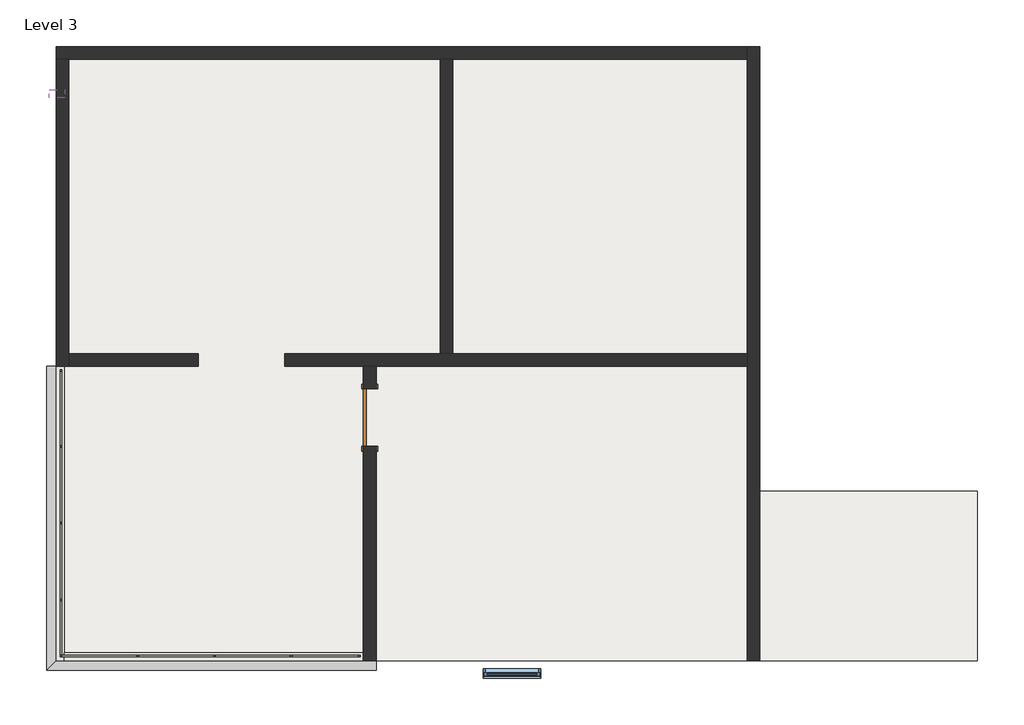
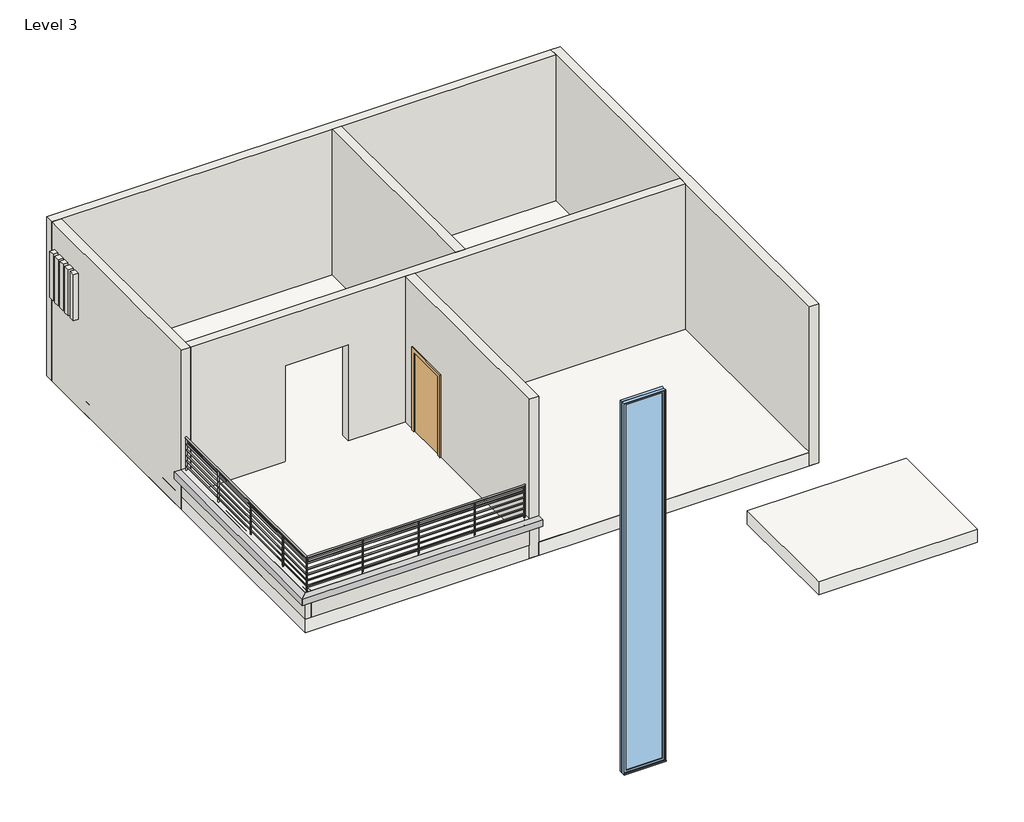
# One storey: 9 walls, 4 roofs, 2 proxies, 1 door, 1 railing, 1 window.
"""IFC4 building model written with IfcOpenShell, lengths in millimetres."""

from ifc_helpers import new_model, si_unit, point, frame, frame_2d, origin, place, context, project, spatial, polyline, circle_curve, ellipse_curve, trimmed, segment, composite_curve, outline, extrude, faceted_brep, transform, mapped, element, save
from ifc_brep_helpers import plane_surface, cylinder_surface, advanced_brep
from components import door_54dd4da4, walls_4_walls_4_d362682a, window_9b859ad1

model = new_model("IFC4")

# Units and contexts
model_context = context("Model", 3, world=origin())
ifc_project = project(units=[si_unit("LENGTHUNIT", "METRE", prefix="MILLI")], contexts=[model_context])

# Site, building, storey
site = spatial("IfcSite", under=ifc_project)
building = spatial("IfcBuilding", under=site)
storey = spatial("IfcBuildingStorey", under=building, Name="Level 3", Elevation=7315.2)

# Proxies
placement = place(None, origin())
element("IfcBuildingElementProxy", 1, Name="Cornice", ObjectType="Cornice", at=placement, inside=storey, context=model_context, shape_type="SweptSolid", body=[
    extrude(outline(polyline([(-12708.8681702, 4224.2612165), (-12556.4681702, 4224.2612165), (-12556.4681702, -449.3387835), (-12708.8681702, -601.7387835), (-12708.8681702, 4224.2612165)])), frame((0.0, 0.0, 8077.2), z_axis=(0.0, 0.0, 1.0), x_axis=(1.0, 0.0, 0.0)), (0.0, 0.0, 1.0), 152.4),
])
element("IfcBuildingElementProxy", 2, Name="Cornice", ObjectType="Cornice", at=placement, inside=storey, context=model_context, shape_type="SweptSolid", body=[
    extrude(outline(polyline([(-12708.8681702, -601.7387835), (-12556.4681702, -449.3387835), (-7476.4681702, -449.3387835), (-7476.4681702, -601.7387835), (-12708.8681702, -601.7387835)])), frame((0.0, 0.0, 8077.2), z_axis=(0.0, 0.0, 1.0), x_axis=(1.0, 0.0, 0.0)), (0.0, 0.0, 1.0), 152.4),
])

# Door
door_shape = door_54dd4da4(model_context)
element("IfcDoor", 3, ObjectType="Single-Flush : 36\" x 84\"", at=placement, inside=storey, context=model_context, shape_type="MappedRepresentation", body=[
    mapped(door_shape, transform((-7578.0681702, 3411.4612165, 7315.2), x_axis=(0.0, 1.0, 0.0), y_axis=(-1.0, 0.0, 0.0), z_axis=(0.0, 0.0, 1.0))),
])

# Railing
element("IfcRailing", 4, ObjectType="Guardrail - Pipe", at=placement, inside=storey, context=model_context, shape_type="SolidModel", body=[
    advanced_brep(
    [(-12423.1181702, 4173.4612165, 8820.15), (-12385.0181702, 4173.4612165, 8820.15), (-12423.1181702, -315.9887835, 8820.15), (-12385.0181702, -277.8887835, 8820.15), (-7730.4681702, -315.9887835, 8820.15), (-7730.4681702, -277.8887835, 8820.15)],
    [
        (0, 1, circle_curve(frame((-12404.0681702, 4173.4612165, 8820.15), z_axis=(0.0, 1.0, 0.0), x_axis=(1.0, 0.0, 0.0)), 19.05)),
        (1, 0, circle_curve(frame((-12404.0681702, 4173.4612165, 8820.15), z_axis=(0.0, 1.0, 0.0), x_axis=(1.0, 0.0, 0.0)), 19.05)),
        (0, 2),
        (2, 3, ellipse_curve(frame((-12404.0681702, -296.9387835, 8820.15), z_axis=(-0.7071067811865459, 0.7071067811865492, 0.0), x_axis=(0.7071067811865492, 0.7071067811865458, 0.0)), 26.9407684, 19.05)),
        (3, 1),
        (3, 2, ellipse_curve(frame((-12404.0681702, -296.9387835, 8820.15), z_axis=(-0.7071067811865459, 0.7071067811865492, 0.0), x_axis=(0.7071067811865492, 0.7071067811865458, 0.0)), 26.9407684, 19.05)),
        (4, 5, circle_curve(frame((-7730.4681702, -296.9387835, 8820.15), z_axis=(1.0, 0.0, 0.0), x_axis=(0.0, 1.0, 0.0)), 19.05)),
        (5, 4, circle_curve(frame((-7730.4681702, -296.9387835, 8820.15), z_axis=(1.0, 0.0, 0.0), x_axis=(0.0, 1.0, 0.0)), 19.05)),
        (2, 4),
        (5, 3),
    ],
    [
        plane_surface(frame((-12404.0681702, 4173.4612165, 8839.2), z_axis=(0.0, 1.0, 0.0), x_axis=(0.0, 0.0, -1.0))),
        cylinder_surface(frame((-12404.0681702, 4173.4612165, 8820.15), z_axis=(0.0, 1.0, 0.0), x_axis=(1.0, 0.0, 0.0)), 19.05),
        plane_surface(frame((-7730.4681702, -296.9387835, 8839.2), z_axis=(1.0, 0.0, 0.0), x_axis=(0.0, 1.0, 0.0))),
        cylinder_surface(frame((-12404.0681702, -296.9387835, 8820.15), z_axis=(-1.0, 0.0, 0.0), x_axis=(0.0, 1.0, 0.0)), 19.05),
    ],
    [
        (0, [[1, 2]]),
        (1, [[-1, 3, 4, 5]]),
        (1, [[-2, -5, 6, -3]]),
        (2, [[7, 8]]),
        (3, [[-4, 9, -8, 10]]),
        (3, [[-6, -10, -7, -9]]),
    ],
),
    advanced_brep(
    [(-12499.3181702, 4173.4612165, 8972.55), (-12461.2181702, 4173.4612165, 8972.55), (-7730.4681702, -392.1887835, 8972.55), (-7730.4681702, -354.0887835, 8972.55), (-12499.3181702, -392.1887835, 8972.55), (-12461.2181702, -354.0887835, 8972.55)],
    [
        (0, 1, circle_curve(frame((-12480.2681702, 4173.4612165, 8972.55), z_axis=(0.0, 1.0, 0.0), x_axis=(1.0, 0.0, 0.0)), 19.05)),
        (1, 0, circle_curve(frame((-12480.2681702, 4173.4612165, 8972.55), z_axis=(0.0, 1.0, 0.0), x_axis=(1.0, 0.0, 0.0)), 19.05)),
        (2, 3, circle_curve(frame((-7730.4681702, -373.1387835, 8972.55), z_axis=(1.0, 0.0, 0.0), x_axis=(0.0, 1.0, 0.0)), 19.05)),
        (3, 2, circle_curve(frame((-7730.4681702, -373.1387835, 8972.55), z_axis=(1.0, 0.0, 0.0), x_axis=(0.0, 1.0, 0.0)), 19.05)),
        (0, 4),
        (4, 5, ellipse_curve(frame((-12480.2681702, -373.1387835, 8972.55), z_axis=(-0.7071067811865459, 0.7071067811865492, 0.0), x_axis=(0.7071067811865492, 0.7071067811865458, 0.0)), 26.9407684, 19.05)),
        (5, 1),
        (5, 4, ellipse_curve(frame((-12480.2681702, -373.1387835, 8972.55), z_axis=(-0.7071067811865459, 0.7071067811865492, 0.0), x_axis=(0.7071067811865492, 0.7071067811865458, 0.0)), 26.9407684, 19.05)),
        (4, 2),
        (3, 5),
    ],
    [
        plane_surface(frame((-12480.2681702, 4173.4612165, 8991.6), z_axis=(0.0, 1.0, 0.0), x_axis=(0.0, 0.0, -1.0))),
        plane_surface(frame((-7730.4681702, -373.1387835, 8991.6), z_axis=(1.0, 0.0, 0.0), x_axis=(0.0, 1.0, 0.0))),
        cylinder_surface(frame((-12480.2681702, 4173.4612165, 8972.55), z_axis=(0.0, 1.0, 0.0), x_axis=(1.0, 0.0, 0.0)), 19.05),
        cylinder_surface(frame((-12480.2681702, -373.1387835, 8972.55), z_axis=(-1.0, 0.0, 0.0), x_axis=(0.0, 1.0, 0.0)), 19.05),
    ],
    [
        (0, [[1, 2]]),
        (1, [[3, 4]]),
        (2, [[-1, 5, 6, 7]]),
        (2, [[-2, -7, 8, -5]]),
        (3, [[-6, 9, -4, 10]]),
        (3, [[-8, -10, -3, -9]]),
    ],
),
    advanced_brep(
    [(-12467.5681702, 4173.4612165, 8826.5), (-12492.9681702, 4173.4612165, 8826.5), (-7730.4681702, -360.4387835, 8826.5), (-7730.4681702, -385.8387835, 8826.5), (-12467.5681702, -360.4387835, 8826.5), (-12492.9681702, -385.8387835, 8826.5)],
    [
        (0, 1, circle_curve(frame((-12480.2681702, 4173.4612165, 8826.5), z_axis=(0.0, 1.0, 0.0), x_axis=(-1.0, 0.0, 0.0)), 12.7)),
        (1, 0, circle_curve(frame((-12480.2681702, 4173.4612165, 8826.5), z_axis=(0.0, 1.0, 0.0), x_axis=(-1.0, 0.0, 0.0)), 12.7)),
        (2, 3, circle_curve(frame((-7730.4681702, -373.1387835, 8826.5), z_axis=(1.0, 0.0, 0.0), x_axis=(0.0, -1.0, 0.0)), 12.7)),
        (3, 2, circle_curve(frame((-7730.4681702, -373.1387835, 8826.5), z_axis=(1.0, 0.0, 0.0), x_axis=(0.0, -1.0, 0.0)), 12.7)),
        (0, 4),
        (4, 5, ellipse_curve(frame((-12480.2681702, -373.1387835, 8826.5), z_axis=(-0.7071067811865459, 0.7071067811865492, 0.0), x_axis=(0.7071067811865492, 0.7071067811865458, 0.0)), 17.9605122, 12.7)),
        (5, 1),
        (5, 4, ellipse_curve(frame((-12480.2681702, -373.1387835, 8826.5), z_axis=(-0.7071067811865459, 0.7071067811865492, 0.0), x_axis=(0.7071067811865492, 0.7071067811865458, 0.0)), 17.9605122, 12.7)),
        (4, 2),
        (3, 5),
    ],
    [
        plane_surface(frame((-12480.2681702, 4173.4612165, 8839.2), z_axis=(0.0, 1.0, 0.0), x_axis=(0.0, 0.0, -1.0))),
        plane_surface(frame((-7730.4681702, -373.1387835, 8839.2), z_axis=(1.0, 0.0, 0.0), x_axis=(0.0, 1.0, 0.0))),
        cylinder_surface(frame((-12480.2681702, 4173.4612165, 8826.5), z_axis=(0.0, 1.0, 0.0), x_axis=(-1.0, 0.0, 0.0)), 12.7),
        cylinder_surface(frame((-12480.2681702, -373.1387835, 8826.5), z_axis=(-1.0, 0.0, 0.0), x_axis=(0.0, -1.0, 0.0)), 12.7),
    ],
    [
        (0, [[1, 2]]),
        (1, [[3, 4]]),
        (2, [[-1, 5, 6, 7]]),
        (2, [[-2, -7, 8, -5]]),
        (3, [[-6, 9, -4, 10]]),
        (3, [[-8, -10, -3, -9]]),
    ],
),
    advanced_brep(
    [(-12467.5681702, 4173.4612165, 8699.5), (-12492.9681702, 4173.4612165, 8699.5), (-7730.4681702, -360.4387835, 8699.5), (-7730.4681702, -385.8387835, 8699.5), (-12467.5681702, -360.4387835, 8699.5), (-12492.9681702, -385.8387835, 8699.5)],
    [
        (0, 1, circle_curve(frame((-12480.2681702, 4173.4612165, 8699.5), z_axis=(0.0, 1.0, 0.0), x_axis=(-1.0, 0.0, 0.0)), 12.7)),
        (1, 0, circle_curve(frame((-12480.2681702, 4173.4612165, 8699.5), z_axis=(0.0, 1.0, 0.0), x_axis=(-1.0, 0.0, 0.0)), 12.7)),
        (2, 3, circle_curve(frame((-7730.4681702, -373.1387835, 8699.5), z_axis=(1.0, 0.0, 0.0), x_axis=(0.0, -1.0, 0.0)), 12.7)),
        (3, 2, circle_curve(frame((-7730.4681702, -373.1387835, 8699.5), z_axis=(1.0, 0.0, 0.0), x_axis=(0.0, -1.0, 0.0)), 12.7)),
        (0, 4),
        (4, 5, ellipse_curve(frame((-12480.2681702, -373.1387835, 8699.5), z_axis=(-0.7071067811865459, 0.7071067811865492, 0.0), x_axis=(0.7071067811865492, 0.7071067811865458, 0.0)), 17.9605122, 12.7)),
        (5, 1),
        (5, 4, ellipse_curve(frame((-12480.2681702, -373.1387835, 8699.5), z_axis=(-0.7071067811865459, 0.7071067811865492, 0.0), x_axis=(0.7071067811865492, 0.7071067811865458, 0.0)), 17.9605122, 12.7)),
        (4, 2),
        (3, 5),
    ],
    [
        plane_surface(frame((-12480.2681702, 4173.4612165, 8712.2), z_axis=(0.0, 1.0, 0.0), x_axis=(0.0, 0.0, -1.0))),
        plane_surface(frame((-7730.4681702, -373.1387835, 8712.2), z_axis=(1.0, 0.0, 0.0), x_axis=(0.0, 1.0, 0.0))),
        cylinder_surface(frame((-12480.2681702, 4173.4612165, 8699.5), z_axis=(0.0, 1.0, 0.0), x_axis=(-1.0, 0.0, 0.0)), 12.7),
        cylinder_surface(frame((-12480.2681702, -373.1387835, 8699.5), z_axis=(-1.0, 0.0, 0.0), x_axis=(0.0, -1.0, 0.0)), 12.7),
    ],
    [
        (0, [[1, 2]]),
        (1, [[3, 4]]),
        (2, [[-1, 5, 6, 7]]),
        (2, [[-2, -7, 8, -5]]),
        (3, [[-6, 9, -4, 10]]),
        (3, [[-8, -10, -3, -9]]),
    ],
),
    advanced_brep(
    [(-12467.5681702, 4173.4612165, 8572.5), (-12492.9681702, 4173.4612165, 8572.5), (-12467.5681702, -360.4387835, 8572.5), (-12492.9681702, -385.8387835, 8572.5), (-7730.4681702, -360.4387835, 8572.5), (-7730.4681702, -385.8387835, 8572.5)],
    [
        (0, 1, circle_curve(frame((-12480.2681702, 4173.4612165, 8572.5), z_axis=(0.0, 1.0, 0.0), x_axis=(-1.0, 0.0, 0.0)), 12.7)),
        (1, 0, circle_curve(frame((-12480.2681702, 4173.4612165, 8572.5), z_axis=(0.0, 1.0, 0.0), x_axis=(-1.0, 0.0, 0.0)), 12.7)),
        (0, 2),
        (2, 3, ellipse_curve(frame((-12480.2681702, -373.1387835, 8572.5), z_axis=(-0.7071067811865459, 0.7071067811865492, 0.0), x_axis=(0.7071067811865492, 0.7071067811865458, 0.0)), 17.9605122, 12.7)),
        (3, 1),
        (3, 2, ellipse_curve(frame((-12480.2681702, -373.1387835, 8572.5), z_axis=(-0.7071067811865459, 0.7071067811865492, 0.0), x_axis=(0.7071067811865492, 0.7071067811865458, 0.0)), 17.9605122, 12.7)),
        (4, 5, circle_curve(frame((-7730.4681702, -373.1387835, 8572.5), z_axis=(1.0, 0.0, 0.0), x_axis=(0.0, -1.0, 0.0)), 12.7)),
        (5, 4, circle_curve(frame((-7730.4681702, -373.1387835, 8572.5), z_axis=(1.0, 0.0, 0.0), x_axis=(0.0, -1.0, 0.0)), 12.7)),
        (2, 4),
        (5, 3),
    ],
    [
        plane_surface(frame((-12480.2681702, 4173.4612165, 8585.2), z_axis=(0.0, 1.0, 0.0), x_axis=(0.0, 0.0, -1.0))),
        cylinder_surface(frame((-12480.2681702, 4173.4612165, 8572.5), z_axis=(0.0, 1.0, 0.0), x_axis=(-1.0, 0.0, 0.0)), 12.7),
        plane_surface(frame((-7730.4681702, -373.1387835, 8585.2), z_axis=(1.0, 0.0, 0.0), x_axis=(0.0, 1.0, 0.0))),
        cylinder_surface(frame((-12480.2681702, -373.1387835, 8572.5), z_axis=(-1.0, 0.0, 0.0), x_axis=(0.0, -1.0, 0.0)), 12.7),
    ],
    [
        (0, [[1, 2]]),
        (1, [[-1, 3, 4, 5]]),
        (1, [[-2, -5, 6, -3]]),
        (2, [[7, 8]]),
        (3, [[-4, 9, -8, 10]]),
        (3, [[-6, -10, -7, -9]]),
    ],
),
    advanced_brep(
    [(-12467.5681702, 4173.4612165, 8445.5), (-12492.9681702, 4173.4612165, 8445.5), (-12467.5681702, -360.4387835, 8445.5), (-12492.9681702, -385.8387835, 8445.5), (-7730.4681702, -360.4387835, 8445.5), (-7730.4681702, -385.8387835, 8445.5)],
    [
        (0, 1, circle_curve(frame((-12480.2681702, 4173.4612165, 8445.5), z_axis=(0.0, 1.0, 0.0), x_axis=(-1.0, 0.0, 0.0)), 12.7)),
        (1, 0, circle_curve(frame((-12480.2681702, 4173.4612165, 8445.5), z_axis=(0.0, 1.0, 0.0), x_axis=(-1.0, 0.0, 0.0)), 12.7)),
        (0, 2),
        (2, 3, ellipse_curve(frame((-12480.2681702, -373.1387835, 8445.5), z_axis=(-0.7071067811865459, 0.7071067811865492, 0.0), x_axis=(0.7071067811865492, 0.7071067811865458, 0.0)), 17.9605122, 12.7)),
        (3, 1),
        (3, 2, ellipse_curve(frame((-12480.2681702, -373.1387835, 8445.5), z_axis=(-0.7071067811865459, 0.7071067811865492, 0.0), x_axis=(0.7071067811865492, 0.7071067811865458, 0.0)), 17.9605122, 12.7)),
        (4, 5, circle_curve(frame((-7730.4681702, -373.1387835, 8445.5), z_axis=(1.0, 0.0, 0.0), x_axis=(0.0, -1.0, 0.0)), 12.7)),
        (5, 4, circle_curve(frame((-7730.4681702, -373.1387835, 8445.5), z_axis=(1.0, 0.0, 0.0), x_axis=(0.0, -1.0, 0.0)), 12.7)),
        (2, 4),
        (5, 3),
    ],
    [
        plane_surface(frame((-12480.2681702, 4173.4612165, 8458.2), z_axis=(0.0, 1.0, 0.0), x_axis=(0.0, 0.0, -1.0))),
        cylinder_surface(frame((-12480.2681702, 4173.4612165, 8445.5), z_axis=(0.0, 1.0, 0.0), x_axis=(-1.0, 0.0, 0.0)), 12.7),
        plane_surface(frame((-7730.4681702, -373.1387835, 8458.2), z_axis=(1.0, 0.0, 0.0), x_axis=(0.0, 1.0, 0.0))),
        cylinder_surface(frame((-12480.2681702, -373.1387835, 8445.5), z_axis=(-1.0, 0.0, 0.0), x_axis=(0.0, -1.0, 0.0)), 12.7),
    ],
    [
        (0, [[1, 2]]),
        (1, [[-1, 3, 4, 5]]),
        (1, [[-2, -5, 6, -3]]),
        (2, [[7, 8]]),
        (3, [[-4, 9, -8, 10]]),
        (3, [[-6, -10, -7, -9]]),
    ],
),
    advanced_brep(
    [(-12467.5681702, 4173.4612165, 8318.5), (-12492.9681702, 4173.4612165, 8318.5), (-12467.5681702, -360.4387835, 8318.5), (-12492.9681702, -385.8387835, 8318.5), (-7730.4681702, -360.4387835, 8318.5), (-7730.4681702, -385.8387835, 8318.5)],
    [
        (0, 1, circle_curve(frame((-12480.2681702, 4173.4612165, 8318.5), z_axis=(0.0, 1.0, 0.0), x_axis=(-1.0, 0.0, 0.0)), 12.7)),
        (1, 0, circle_curve(frame((-12480.2681702, 4173.4612165, 8318.5), z_axis=(0.0, 1.0, 0.0), x_axis=(-1.0, 0.0, 0.0)), 12.7)),
        (0, 2),
        (2, 3, ellipse_curve(frame((-12480.2681702, -373.1387835, 8318.5), z_axis=(-0.7071067811865459, 0.7071067811865492, 0.0), x_axis=(0.7071067811865492, 0.7071067811865458, 0.0)), 17.9605122, 12.7)),
        (3, 1),
        (3, 2, ellipse_curve(frame((-12480.2681702, -373.1387835, 8318.5), z_axis=(-0.7071067811865459, 0.7071067811865492, 0.0), x_axis=(0.7071067811865492, 0.7071067811865458, 0.0)), 17.9605122, 12.7)),
        (4, 5, circle_curve(frame((-7730.4681702, -373.1387835, 8318.5), z_axis=(1.0, 0.0, 0.0), x_axis=(0.0, -1.0, 0.0)), 12.7)),
        (5, 4, circle_curve(frame((-7730.4681702, -373.1387835, 8318.5), z_axis=(1.0, 0.0, 0.0), x_axis=(0.0, -1.0, 0.0)), 12.7)),
        (2, 4),
        (5, 3),
    ],
    [
        plane_surface(frame((-12480.2681702, 4173.4612165, 8331.2), z_axis=(0.0, 1.0, 0.0), x_axis=(0.0, 0.0, -1.0))),
        cylinder_surface(frame((-12480.2681702, 4173.4612165, 8318.5), z_axis=(0.0, 1.0, 0.0), x_axis=(-1.0, 0.0, 0.0)), 12.7),
        plane_surface(frame((-7730.4681702, -373.1387835, 8331.2), z_axis=(1.0, 0.0, 0.0), x_axis=(0.0, 1.0, 0.0))),
        cylinder_surface(frame((-12480.2681702, -373.1387835, 8318.5), z_axis=(-1.0, 0.0, 0.0), x_axis=(0.0, -1.0, 0.0)), 12.7),
    ],
    [
        (0, [[1, 2]]),
        (1, [[-1, 3, 4, 5]]),
        (1, [[-2, -5, 6, -3]]),
        (2, [[7, 8]]),
        (3, [[-4, 9, -8, 10]]),
        (3, [[-6, -10, -7, -9]]),
    ],
),
    advanced_brep(
    [(-12467.5681702, 4173.4612165, 8191.5), (-12492.9681702, 4173.4612165, 8191.5), (-12467.5681702, -360.4387835, 8191.5), (-12492.9681702, -385.8387835, 8191.5), (-7730.4681702, -360.4387835, 8191.5), (-7730.4681702, -385.8387835, 8191.5)],
    [
        (0, 1, circle_curve(frame((-12480.2681702, 4173.4612165, 8191.5), z_axis=(0.0, 1.0, 0.0), x_axis=(-1.0, 0.0, 0.0)), 12.7)),
        (1, 0, circle_curve(frame((-12480.2681702, 4173.4612165, 8191.5), z_axis=(0.0, 1.0, 0.0), x_axis=(-1.0, 0.0, 0.0)), 12.7)),
        (0, 2),
        (2, 3, ellipse_curve(frame((-12480.2681702, -373.1387835, 8191.5), z_axis=(-0.7071067811865459, 0.7071067811865492, 0.0), x_axis=(0.7071067811865492, 0.7071067811865458, 0.0)), 17.9605122, 12.7)),
        (3, 1),
        (3, 2, ellipse_curve(frame((-12480.2681702, -373.1387835, 8191.5), z_axis=(-0.7071067811865459, 0.7071067811865492, 0.0), x_axis=(0.7071067811865492, 0.7071067811865458, 0.0)), 17.9605122, 12.7)),
        (4, 5, circle_curve(frame((-7730.4681702, -373.1387835, 8191.5), z_axis=(1.0, 0.0, 0.0), x_axis=(0.0, -1.0, 0.0)), 12.7)),
        (5, 4, circle_curve(frame((-7730.4681702, -373.1387835, 8191.5), z_axis=(1.0, 0.0, 0.0), x_axis=(0.0, -1.0, 0.0)), 12.7)),
        (2, 4),
        (5, 3),
    ],
    [
        plane_surface(frame((-12480.2681702, 4173.4612165, 8204.2), z_axis=(0.0, 1.0, 0.0), x_axis=(0.0, 0.0, -1.0))),
        cylinder_surface(frame((-12480.2681702, 4173.4612165, 8191.5), z_axis=(0.0, 1.0, 0.0), x_axis=(-1.0, 0.0, 0.0)), 12.7),
        plane_surface(frame((-7730.4681702, -373.1387835, 8204.2), z_axis=(1.0, 0.0, 0.0), x_axis=(0.0, 1.0, 0.0))),
        cylinder_surface(frame((-12480.2681702, -373.1387835, 8191.5), z_axis=(-1.0, 0.0, 0.0), x_axis=(0.0, -1.0, 0.0)), 12.7),
    ],
    [
        (0, [[1, 2]]),
        (1, [[-1, 3, 4, 5]]),
        (1, [[-2, -5, 6, -3]]),
        (2, [[7, 8]]),
        (3, [[-4, 9, -8, 10]]),
        (3, [[-6, -10, -7, -9]]),
    ],
),
    advanced_brep(
    [(-12467.5681702, 4173.4612165, 8064.5), (-12492.9681702, 4173.4612165, 8064.5), (-12467.5681702, -360.4387835, 8064.5), (-12492.9681702, -385.8387835, 8064.5), (-7730.4681702, -360.4387835, 8064.5), (-7730.4681702, -385.8387835, 8064.5)],
    [
        (0, 1, circle_curve(frame((-12480.2681702, 4173.4612165, 8064.5), z_axis=(0.0, 1.0, 0.0), x_axis=(-1.0, 0.0, 0.0)), 12.7)),
        (1, 0, circle_curve(frame((-12480.2681702, 4173.4612165, 8064.5), z_axis=(0.0, 1.0, 0.0), x_axis=(-1.0, 0.0, 0.0)), 12.7)),
        (0, 2),
        (2, 3, ellipse_curve(frame((-12480.2681702, -373.1387835, 8064.5), z_axis=(-0.7071067811865459, 0.7071067811865492, 0.0), x_axis=(0.7071067811865492, 0.7071067811865458, 0.0)), 17.9605122, 12.7)),
        (3, 1),
        (3, 2, ellipse_curve(frame((-12480.2681702, -373.1387835, 8064.5), z_axis=(-0.7071067811865459, 0.7071067811865492, 0.0), x_axis=(0.7071067811865492, 0.7071067811865458, 0.0)), 17.9605122, 12.7)),
        (4, 5, circle_curve(frame((-7730.4681702, -373.1387835, 8064.5), z_axis=(1.0, 0.0, 0.0), x_axis=(0.0, -1.0, 0.0)), 12.7)),
        (5, 4, circle_curve(frame((-7730.4681702, -373.1387835, 8064.5), z_axis=(1.0, 0.0, 0.0), x_axis=(0.0, -1.0, 0.0)), 12.7)),
        (2, 4),
        (5, 3),
    ],
    [
        plane_surface(frame((-12480.2681702, 4173.4612165, 8077.2), z_axis=(0.0, 1.0, 0.0), x_axis=(0.0, 0.0, -1.0))),
        cylinder_surface(frame((-12480.2681702, 4173.4612165, 8064.5), z_axis=(0.0, 1.0, 0.0), x_axis=(-1.0, 0.0, 0.0)), 12.7),
        plane_surface(frame((-7730.4681702, -373.1387835, 8077.2), z_axis=(1.0, 0.0, 0.0), x_axis=(0.0, 1.0, 0.0))),
        cylinder_surface(frame((-12480.2681702, -373.1387835, 8064.5), z_axis=(-1.0, 0.0, 0.0), x_axis=(0.0, -1.0, 0.0)), 12.7),
    ],
    [
        (0, [[1, 2]]),
        (1, [[-1, 3, 4, 5]]),
        (1, [[-2, -5, 6, -3]]),
        (2, [[7, 8]]),
        (3, [[-4, 9, -8, 10]]),
        (3, [[-6, -10, -7, -9]]),
    ],
),
    extrude(outline(composite_curve([segment(trimmed(circle_curve(frame_2d((-8822.6681702, -373.1387835)), 12.7), [point((-8822.6681702, -360.4387835))], [point((-8822.6681702, -385.8387835))], False, "CARTESIAN"), True, "CONTINUOUS"), segment(trimmed(circle_curve(frame_2d((-8822.6681702, -373.1387835)), 12.7), [point((-8822.6681702, -385.8387835))], [point((-8822.6681702, -360.4387835))], False, "CARTESIAN"), True, "CONTINUOUS")], self_intersect=False)), frame((0.0, 0.0, 7924.8), z_axis=(0.0, 0.0, 1.0), x_axis=(1.0, 0.0, 0.0)), (0.0, 0.0, 1.0), 1028.7),
    extrude(outline(composite_curve([segment(trimmed(circle_curve(frame_2d((-10041.8681702, -373.1387835)), 12.7), [point((-10041.8681702, -360.4387835))], [point((-10041.8681702, -385.8387835))], False, "CARTESIAN"), True, "CONTINUOUS"), segment(trimmed(circle_curve(frame_2d((-10041.8681702, -373.1387835)), 12.7), [point((-10041.8681702, -385.8387835))], [point((-10041.8681702, -360.4387835))], False, "CARTESIAN"), True, "CONTINUOUS")], self_intersect=False)), frame((0.0, 0.0, 7924.8), z_axis=(0.0, 0.0, 1.0), x_axis=(1.0, 0.0, 0.0)), (0.0, 0.0, 1.0), 1028.7),
    extrude(outline(composite_curve([segment(trimmed(circle_curve(frame_2d((-11261.0681702, -373.1387835)), 12.7), [point((-11261.0681702, -360.4387835))], [point((-11261.0681702, -385.8387835))], False, "CARTESIAN"), True, "CONTINUOUS"), segment(trimmed(circle_curve(frame_2d((-11261.0681702, -373.1387835)), 12.7), [point((-11261.0681702, -385.8387835))], [point((-11261.0681702, -360.4387835))], False, "CARTESIAN"), True, "CONTINUOUS")], self_intersect=False)), frame((0.0, 0.0, 7924.8), z_axis=(0.0, 0.0, 1.0), x_axis=(1.0, 0.0, 0.0)), (0.0, 0.0, 1.0), 1028.7),
    extrude(outline(composite_curve([segment(trimmed(circle_curve(frame_2d((-12480.2681702, 515.8612165)), 12.7), [point((-12467.5681702, 515.8612165))], [point((-12492.9681702, 515.8612165))], False, "CARTESIAN"), True, "CONTINUOUS"), segment(trimmed(circle_curve(frame_2d((-12480.2681702, 515.8612165)), 12.7), [point((-12492.9681702, 515.8612165))], [point((-12467.5681702, 515.8612165))], False, "CARTESIAN"), True, "CONTINUOUS")], self_intersect=False)), frame((0.0, 0.0, 7924.8), z_axis=(0.0, 0.0, 1.0), x_axis=(1.0, 0.0, 0.0)), (0.0, 0.0, 1.0), 1028.7),
    extrude(outline(composite_curve([segment(trimmed(circle_curve(frame_2d((-12480.2681702, 1735.0612165)), 12.7), [point((-12467.5681702, 1735.0612165))], [point((-12492.9681702, 1735.0612165))], False, "CARTESIAN"), True, "CONTINUOUS"), segment(trimmed(circle_curve(frame_2d((-12480.2681702, 1735.0612165)), 12.7), [point((-12492.9681702, 1735.0612165))], [point((-12467.5681702, 1735.0612165))], False, "CARTESIAN"), True, "CONTINUOUS")], self_intersect=False)), frame((0.0, 0.0, 7924.8), z_axis=(0.0, 0.0, 1.0), x_axis=(1.0, 0.0, 0.0)), (0.0, 0.0, 1.0), 1028.7),
    extrude(outline(composite_curve([segment(trimmed(circle_curve(frame_2d((-12480.2681702, 2954.2612165)), 12.7), [point((-12467.5681702, 2954.2612165))], [point((-12492.9681702, 2954.2612165))], False, "CARTESIAN"), True, "CONTINUOUS"), segment(trimmed(circle_curve(frame_2d((-12480.2681702, 2954.2612165)), 12.7), [point((-12492.9681702, 2954.2612165))], [point((-12467.5681702, 2954.2612165))], False, "CARTESIAN"), True, "CONTINUOUS")], self_intersect=False)), frame((0.0, 0.0, 7924.8), z_axis=(0.0, 0.0, 1.0), x_axis=(1.0, 0.0, 0.0)), (0.0, 0.0, 1.0), 1028.7),
    extrude(outline(composite_curve([segment(trimmed(circle_curve(frame_2d((-12480.2681702, -373.1387835)), 12.7), [point((-12467.5681702, -373.1387835))], [point((-12492.9681702, -373.1387835))], False, "CARTESIAN"), True, "CONTINUOUS"), segment(trimmed(circle_curve(frame_2d((-12480.2681702, -373.1387835)), 12.7), [point((-12492.9681702, -373.1387835))], [point((-12467.5681702, -373.1387835))], False, "CARTESIAN"), True, "CONTINUOUS")], self_intersect=False)), frame((0.0, 0.0, 7924.8), z_axis=(0.0, 0.0, 1.0), x_axis=(1.0, 0.0, 0.0)), (0.0, 0.0, 1.0), 1028.7),
    extrude(outline(composite_curve([segment(trimmed(circle_curve(frame_2d((-7743.1681702, -373.1387835)), 12.7), [point((-7743.1681702, -360.4387835))], [point((-7743.1681702, -385.8387835))], False, "CARTESIAN"), True, "CONTINUOUS"), segment(trimmed(circle_curve(frame_2d((-7743.1681702, -373.1387835)), 12.7), [point((-7743.1681702, -385.8387835))], [point((-7743.1681702, -360.4387835))], False, "CARTESIAN"), True, "CONTINUOUS")], self_intersect=False)), frame((0.0, 0.0, 7924.8), z_axis=(0.0, 0.0, 1.0), x_axis=(1.0, 0.0, 0.0)), (0.0, 0.0, 1.0), 1028.7),
    extrude(outline(composite_curve([segment(trimmed(circle_curve(frame_2d((-12480.2681702, 4160.7612165)), 12.7), [point((-12467.5681702, 4160.7612165))], [point((-12492.9681702, 4160.7612165))], False, "CARTESIAN"), True, "CONTINUOUS"), segment(trimmed(circle_curve(frame_2d((-12480.2681702, 4160.7612165)), 12.7), [point((-12492.9681702, 4160.7612165))], [point((-12467.5681702, 4160.7612165))], False, "CARTESIAN"), True, "CONTINUOUS")], self_intersect=False)), frame((0.0, 0.0, 7924.8), z_axis=(0.0, 0.0, 1.0), x_axis=(1.0, 0.0, 0.0)), (0.0, 0.0, 1.0), 1028.7),
])

# Roofs
element("IfcRoof", 5, ObjectType="Generic - 12\"", at=placement, inside=storey, context=model_context, shape_type="SweptSolid", body=[
    extrude(outline(polyline([(-12556.4681702, 9304.2612165), (-1380.4681702, 9304.2612165), (-1380.4681702, -449.3387835), (-12556.4681702, -449.3387835), (-12556.4681702, 9304.2612165)])), frame((0.0, 0.0, 7315.2), z_axis=(0.0, 0.0, 1.0), x_axis=(1.0, 0.0, 0.0)), (0.0, 0.0, 1.0), 304.8),
])
element("IfcRoof", 6, ObjectType="Generic - 12\"", at=placement, inside=storey, context=model_context, shape_type="SweptSolid", body=[
    extrude(outline(polyline([(-12353.2681702, 9101.0612165), (-1583.6681702, 9101.0612165), (-1583.6681702, -449.3387835), (-7476.4681702, -449.3387835), (-7476.4681702, 4224.2612165), (-7476.4681702, 4376.6612165), (-12353.2681702, 4376.6612165), (-12353.2681702, 9101.0612165)])), frame((0.0, 0.0, 7315.2), z_axis=(0.0, 0.0, 1.0), x_axis=(1.0, 0.0, 0.0)), (0.0, 0.0, 1.0), 304.8),
])
element("IfcRoof", 7, ObjectType="Generic - 12\"", at=placement, inside=storey, context=model_context, shape_type="SweptSolid", body=[
    extrude(outline(polyline([(-12353.2681702, 9101.0612165), (-1583.6681702, 9101.0612165), (-1583.6681702, -449.3387835), (-7476.4681702, -449.3387835), (-7476.4681702, 4427.4612165), (-12353.2681702, 4427.4612165), (-12353.2681702, 9101.0612165)])), frame((0.0, 0.0, 7315.2), z_axis=(0.0, 0.0, 1.0), x_axis=(1.0, 0.0, 0.0)), (0.0, 0.0, 1.0), 304.8),
])
element("IfcRoof", 8, ObjectType="Generic - 12\"", at=placement, inside=storey, context=model_context, shape_type="SweptSolid", body=[
    extrude(outline(polyline([(-1380.4681702, 2243.0612165), (2073.9318298, 2243.0612165), (2073.9318298, -449.3387835), (-1380.4681702, -449.3387835), (-1380.4681702, 2243.0612165)])), frame((0.0, 0.0, 4267.2), z_axis=(0.0, 0.0, 1.0), x_axis=(1.0, 0.0, 0.0)), (0.0, 0.0, 1.0), 304.8),
])

# Walls
element("IfcWall", 9, ObjectType="Generic - 5\"", at=placement, inside=storey, context=model_context, shape_type="Brep", body=[
    faceted_brep([(-12556.4681702, 4224.2612165, 7620.0), (-12556.4681702, -449.3387835, 7620.0), (-12556.4681702, -449.3387835, 8229.6), (-12556.4681702, 4224.2612165, 8229.6), (-12429.4681702, 4224.2612165, 7620.0), (-12429.4681702, 4224.2612165, 8229.6), (-12429.4681702, -322.3387835, 8229.6), (-12429.4681702, -449.3387835, 8229.6), (-12429.4681702, -449.3387835, 7620.0), (-12429.4681702, -322.3387835, 7620.0)], [[[0, 1, 2, 3]], [[4, 5, 6, 7, 8, 9]], [[1, 0, 4, 9, 8]], [[3, 2, 7, 6, 5]], [[2, 1, 8, 7]], [[0, 3, 5, 4]]]),
])
element("IfcWall", 10, ObjectType="Generic - 5\"", at=placement, inside=storey, context=model_context, shape_type="Brep", body=[
    faceted_brep([(-12429.4681702, -449.3387835, 7620.0), (-7679.6681702, -449.3387835, 7620.0), (-7679.6681702, -449.3387835, 8077.2), (-7679.6681702, -449.3387835, 8229.6), (-12429.4681702, -449.3387835, 8229.6), (-12429.4681702, -449.3387835, 8077.2), (-7679.6681702, -322.3387835, 7620.0), (-12429.4681702, -322.3387835, 7620.0), (-12429.4681702, -322.3387835, 8229.6), (-7679.6681702, -322.3387835, 8229.6)], [[[0, 1, 2, 3, 4, 5]], [[6, 7, 8, 9]], [[1, 0, 7, 6]], [[4, 3, 9, 8]], [[4, 8, 7, 0, 5]], [[1, 6, 9, 3, 2]]]),
])
element("IfcWall", 11, ObjectType="Generic - 8\"", at=placement, inside=storey, context=model_context, shape_type="Brep", body=[
    faceted_brep([(-12556.4681702, 9101.0612165, 7315.2), (-12353.2681702, 9101.0612165, 7315.2), (-6460.4681702, 9101.0612165, 7315.2), (-6257.2681702, 9101.0612165, 7315.2), (-1583.6681702, 9101.0612165, 7315.2), (-1583.6681702, 9101.0612165, 10972.8), (-6257.2681702, 9101.0612165, 10972.8), (-6460.4681702, 9101.0612165, 10972.8), (-12353.2681702, 9101.0612165, 10972.8), (-12556.4681702, 9101.0612165, 10972.8), (-12556.4681702, 9304.2612165, 7315.2), (-12556.4681702, 9304.2612165, 10972.8), (-1583.6681702, 9304.2612165, 10972.8), (-1583.6681702, 9304.2612165, 7315.2)], [[[0, 1, 2, 3, 4, 5, 6, 7, 8, 9]], [[10, 11, 12, 13]], [[4, 3, 2, 1, 0, 10, 13]], [[0, 9, 11, 10]], [[5, 4, 13, 12]], [[9, 8, 7, 6, 5, 12, 11]]]),
])
element("IfcWall", 12, ObjectType="Generic - 8\"", at=placement, inside=storey, context=model_context, shape_type="Brep", body=[
    faceted_brep([(-12353.2681702, 4224.2612165, 10972.8), (-12353.2681702, 4224.2612165, 7315.2), (-12353.2681702, 4427.4612165, 7315.2), (-12353.2681702, 9101.0612165, 7315.2), (-12353.2681702, 9101.0612165, 10972.8), (-12353.2681702, 4427.4612165, 10972.8), (-12556.4681702, 4224.2612165, 7315.2), (-12556.4681702, 4224.2612165, 7620.0), (-12556.4681702, 4224.2612165, 8229.6), (-12556.4681702, 4224.2612165, 10972.8), (-12556.4681702, 9101.0612165, 10972.8), (-12556.4681702, 9101.0612165, 7315.2)], [[[0, 1, 2, 3, 4, 5]], [[6, 7, 8, 9, 10, 11]], [[3, 2, 1, 6, 11]], [[4, 3, 11, 10]], [[0, 5, 4, 10, 9]], [[0, 9, 8, 7, 6, 1]]]),
])
element("IfcWall", 13, ObjectType="Generic - 8\"", at=placement, inside=storey, context=model_context, shape_type="Brep", body=[
    faceted_brep([(-1583.6681702, 9304.2612165, 7315.2), (-1583.6681702, 9101.0612165, 7315.2), (-1583.6681702, 4427.4612165, 7315.2), (-1583.6681702, 4224.2612165, 7315.2), (-1583.6681702, -449.3387835, 7315.2), (-1583.6681702, -449.3387835, 10972.8), (-1583.6681702, 4224.2612165, 10972.8), (-1583.6681702, 4427.4612165, 10972.8), (-1583.6681702, 9101.0612165, 10972.8), (-1583.6681702, 9304.2612165, 10972.8), (-1380.4681702, 9304.2612165, 7315.2), (-1380.4681702, 9304.2612165, 10972.8), (-1380.4681702, -449.3387835, 10972.8), (-1380.4681702, -449.3387835, 7315.2)], [[[0, 1, 2, 3, 4, 5, 6, 7, 8, 9]], [[10, 11, 12, 13]], [[4, 3, 2, 1, 0, 10, 13]], [[0, 9, 11, 10]], [[5, 4, 13, 12]], [[9, 8, 7, 6, 5, 12, 11]]]),
])
element("IfcWall", 14, ObjectType="Generic - 8\"", at=placement, inside=storey, context=model_context, shape_type="Brep", body=[
    faceted_brep([(-7679.6681702, 4224.2612165, 7315.2), (-7679.6681702, 3868.6612165, 7315.2), (-7679.6681702, 3868.6612165, 9448.8), (-7679.6681702, 2954.2612165, 9448.8), (-7679.6681702, 2954.2612165, 7315.2), (-7679.6681702, -449.3387835, 7315.2), (-7679.6681702, -449.3387835, 7620.0), (-7679.6681702, -449.3387835, 8229.6), (-7679.6681702, -449.3387835, 10972.8), (-7679.6681702, 4224.2612165, 10972.8), (-7476.4681702, 3868.6612165, 9448.8), (-7476.4681702, 3868.6612165, 7315.2), (-7476.4681702, 4224.2612165, 7315.2), (-7476.4681702, 4224.2612165, 10972.8), (-7476.4681702, -449.3387835, 10972.8), (-7476.4681702, -449.3387835, 7315.2), (-7476.4681702, 2954.2612165, 7315.2), (-7476.4681702, 2954.2612165, 9448.8)], [[[0, 1, 2, 3, 4, 5, 6, 7, 8, 9]], [[10, 11, 12, 13, 14, 15, 16, 17]], [[12, 11, 1, 0]], [[16, 15, 5, 4]], [[0, 9, 13, 12]], [[9, 8, 14, 13]], [[5, 15, 14, 8, 7, 6]], [[2, 1, 11, 10]], [[3, 2, 10, 17]], [[4, 3, 17, 16]]]),
])
element("IfcWall", 15, ObjectType="Generic - 8\"", at=placement, inside=storey, context=model_context, shape_type="Brep", body=[
    faceted_brep([(-12353.2681702, 4224.2612165, 10972.8), (-12353.2681702, 4224.2612165, 7315.2), (-10297.0751994, 4224.2612165, 7315.2), (-10297.0751994, 4224.2612165, 9829.8), (-8925.4751994, 4224.2612165, 9829.8), (-8925.4751994, 4224.2612165, 7315.2), (-7679.6681702, 4224.2612165, 7315.2), (-7476.4681702, 4224.2612165, 7315.2), (-1583.6681702, 4224.2612165, 7315.2), (-1583.6681702, 4224.2612165, 10972.8), (-7476.4681702, 4224.2612165, 10972.8), (-7679.6681702, 4224.2612165, 10972.8), (-12353.2681702, 4427.4612165, 7315.2), (-12353.2681702, 4427.4612165, 10972.8), (-6460.4681702, 4427.4612165, 10972.8), (-6257.2681702, 4427.4612165, 10972.8), (-1583.6681702, 4427.4612165, 10972.8), (-1583.6681702, 4427.4612165, 7315.2), (-6257.2681702, 4427.4612165, 7315.2), (-6460.4681702, 4427.4612165, 7315.2), (-8925.4751994, 4427.4612165, 7315.2), (-8925.4751994, 4427.4612165, 9829.8), (-10297.0751994, 4427.4612165, 9829.8), (-10297.0751994, 4427.4612165, 7315.2)], [[[0, 1, 2, 3, 4, 5, 6, 7, 8, 9, 10, 11]], [[12, 13, 14, 15, 16, 17, 18, 19, 20, 21, 22, 23]], [[9, 8, 17, 16]], [[0, 13, 12, 1]], [[0, 11, 10, 9, 16, 15, 14, 13]], [[2, 1, 12, 23]], [[3, 2, 23, 22]], [[4, 3, 22, 21]], [[5, 4, 21, 20]], [[8, 7, 6, 5, 20, 19, 18, 17]]]),
])
element("IfcWall", 16, ObjectType="Generic - 8\"", at=placement, inside=storey, context=model_context, shape_type="SweptSolid", body=[
    extrude(outline(polyline([(-6460.4681702, 4427.4612165), (-6460.4681702, 9101.0612165), (-6257.2681702, 9101.0612165), (-6257.2681702, 4427.4612165), (-6460.4681702, 4427.4612165)])), frame((0.0, 0.0, 7315.2), z_axis=(0.0, 0.0, 1.0), x_axis=(1.0, 0.0, 0.0)), (0.0, 0.0, 1.0), 3657.6),
])
walls_4_walls_4_shape = walls_4_walls_4_d362682a(model_context)
element("IfcWall", 17, ObjectType="Walls 4 : Walls 4", at=placement, inside=storey, context=model_context, shape_type="MappedRepresentation", body=[
    mapped(walls_4_walls_4_shape, transform((0.0, 0.0, 0.0), x_axis=(1.0, 0.0, 0.0), y_axis=(0.0, 1.0, 0.0), z_axis=(0.0, 0.0, 1.0))),
])

# Window
window_shape = window_9b859ad1(model_context)
element("IfcWindow", 18, ObjectType="Instance - Fixed : 36\" x 336\"", at=placement, inside=storey, context=model_context, shape_type="MappedRepresentation", body=[
    mapped(window_shape, transform((-5355.5681702, -639.8387835, 914.4), x_axis=(-1.0, 0.0, 0.0), y_axis=(0.0, -1.0, 0.0), z_axis=(0.0, 0.0, 1.0))),
])

save(model, "model.ifc")

# Revit data of these elements
# Type "Single-Flush : 36\" x 84\""
#   Type Mark = "1"
#   Construction Type Id = "MDOOR"
#   Assembly Code = "C1020"
#   Analytic Construction = "Metal"
#   Thickness = 0' - 2"
#   Heat Transfer Coefficient (U) = 0.651978 BTU/(h·ft²·°F)
#   Height = 7' - 0"
#   Trim Projection Ext = 0' - 1"
#   Trim Projection Int = 0' - 1"
#   Trim Width = 0' - 3"
#   Width = 3' - 0"
#   Define Thermal Properties by = 1
#   Door Material = Door - Panel
#   Frame Material = Door - Frame
#   Visual Light Transmittance = 0
#   Solar Heat Gain Coefficient = 0
#   Function = (empty or 0)
#   Wall Closure = (empty or 0)
# Type "Guardrail - Pipe"
#   Assembly Code = "C2010400"
#   built-in parameter 1008612 = 0.0416667 (stored number, unit not read)
#   built-in parameter 1008611 = 0.0833333 (stored number, unit not read)
#   built-in parameter 1008609 = 4 (stored number, unit not read)
#   built-in parameter 1008604 = 0.166667 (stored number, unit not read)
#   built-in parameter 1008603 = 0.166667 (stored number, unit not read)
#   Railing Height = 3' - 6"
#   built-in parameter 1008630 = 2
#   built-in parameter 1008610 = 1
#   built-in parameter 1008605 = 1
#   built-in parameter 1008618 = Baluster - Round : 1"
# Type "Generic - 12\""
#   Assembly Code = "B1020"
#   Layers, outside or top first: 1' - 0" no material (function 1)
# Type "Generic - 5\""
#   Assembly Code = "B2010"
#   Layers, outside or top first: 0' - 5" no material (function 1)
# Type "Generic - 8\""
#   Assembly Code = "B2010"
#   Layers, outside or top first: 0' - 8" no material (function 1)
# Type "Instance - Fixed : 36\" x 336\""
#   Type Mark = "10"
#   Construction Type Id = "GSP4R"
#   Assembly Code = "B2020100"
#   Analytic Construction = "1/8 in Pilkington single glazing"
#   Visual Light Transmittance = 0.9
#   Thermal Resistance (R) = 0.8466 (h·ft²·°F)/BTU
#   Solar Heat Gain Coefficient = 0.86
#   Heat Transfer Coefficient (U) = 1.1812 BTU/(h·ft²·°F)
#   Height [instance default] = 4' - 0"
#   Default Sill Height = 3' - 0"
#   Width [instance default] = 2' - 0"
#   Window Inset = 0' - 0 3/4"
#   Define Thermal Properties by = 1
#   Glass Pane Material = Glass
#   Sash Material = Sash
#   Wall Closure = (empty or 0)
# Elements 1, 2 (IfcBuildingElementProxy, "Cornice")
#   Phase Created = New Construction
#   Materials on its faces: "Default Wall"
# Element 3 (IfcDoor, "Single-Flush : 36\" x 84\"")
#   Phase Created = New Construction
#   Materials on its faces: "Door - Frame", "Door - Panel"
# Element 4 (IfcRailing, "Guardrail - Pipe")
#   built-in parameter 1008621 = 2 (stored number, unit not read)
#   Phase Created = New Construction
# Elements 5, 6, 7 (IfcRoof, "Generic - 12\"")
#   built-in parameter 1001705 = 25 (stored number, unit not read)
#   built-in parameter 1001710 = 33615
#   Phase Created = New Construction
#   Materials on its faces: "Default Roof"
# Element 8 (IfcRoof, "Generic - 12\"")
#   built-in parameter 1001705 = 15 (stored number, unit not read)
#   built-in parameter 1001701 = -10 (stored number, unit not read)
#   built-in parameter 1001710 = 33615
#   Phase Created = New Construction
#   Materials on its faces: "Default Roof"
# Elements 9, 10 (IfcWall, "Generic - 5\"")
#   built-in parameter 1001111 = 1' - 0"
#   Top Offset = -9' - 0"
#   Base Offset = 1' - 0"
#   wall height = 2' - 0"
#   Phase Created = New Construction
#   Base Constraint = Level 3
#   Top Constraint = Level 4
#   Materials on its faces: "Default Wall"
# Elements 11, 12, 13, 14, 15, 16 (IfcWall, "Generic - 8\"")
#   Top Offset = 0' - 0"
#   Base Offset = 0' - 0"
#   Unconnected Height = 12' - 0"
#   wall height = 12' - 0"
#   Phase Created = New Construction
#   Base Constraint = Level 3
#   Materials on its faces: "Default Wall"
# Element 17 (IfcWall, "Walls 4 : Walls 4")
#   Phase Created = New Construction
#   Materials on its faces: "Default Wall"
# Element 18 (IfcWindow, "Instance - Fixed : 36\" x 336\"")
#   Mark = "1"
#   Width = 3' - 0"
#   Height = 28' - 0"
#   Phase Created = New Construction
#   Materials on its faces: "Sash", "Glass"
# Materials
#   "Door - Panel": class "Wood", colour RGB 210 159 95, transparency 0
#   "Door - Frame": colour RGB 118 70 51, transparency 0
#   "Glass": class "Glass", colour RGB 0 128 192, transparency 0.75, Description = "Soda Lime Glass", Cost = 0
#   "Sash": class "Wood", colour RGB 224 178 126, transparency 0
#   "Default Wall": colour RGB 128 128 128, transparency 0
#   "Default Roof": colour RGB 88 101 114, transparency 0
